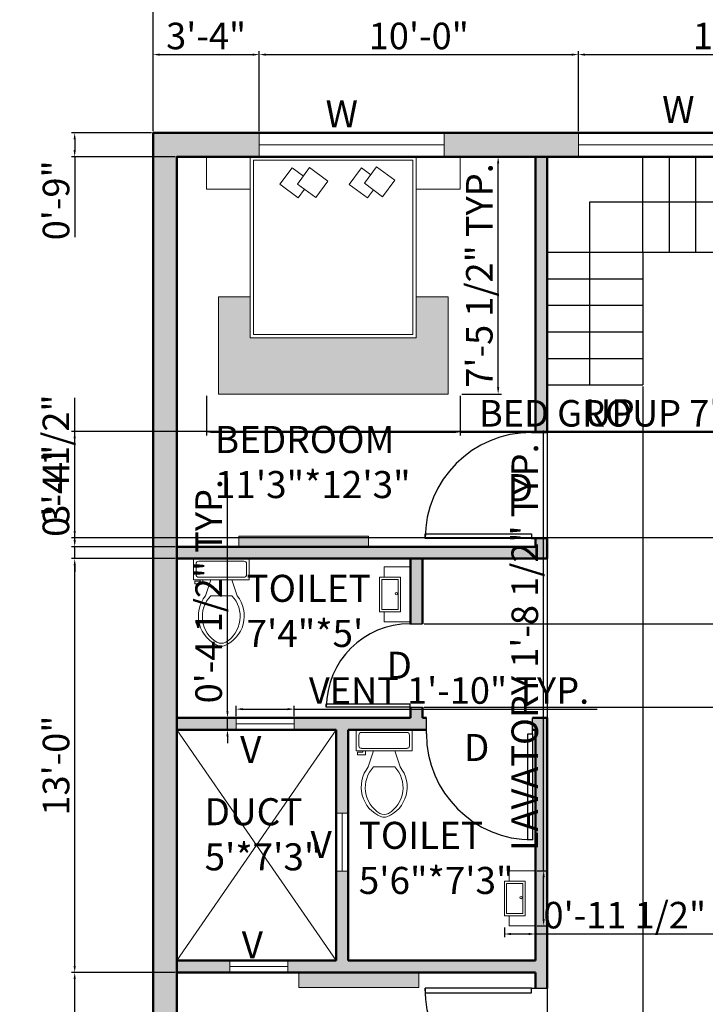
# Model space of a CAD drawing. Units: inches. Extents: x 1822 to 2392, y 2066 to 2908.
# Tile 2 of 4: x 1822 to 2080, y 2256 to 2627. Entities that reach past the tile are written whole.
import ezdxf

# ---------------------------------------------------------------- set-up
doc = ezdxf.new("R2010")
doc.units = ezdxf.units.IN
for name, color, linetype, lineweight in [('A-ANNO-DIMS', 2, 'Continuous', 18), ('A-AREA-IDEN', 83, 'Continuous', 25), ('A-EQPM-PATT', 89, 'Continuous', 13), ('A-FLOR-OPEN', 8, 'Continuous', 18), ('A-FLOR-PATT', 9, 'Continuous', 13), ('A-WALL-PATT', 252, 'Continuous', 13), ('BEDS', 40, 'Continuous', 18), ('DOOR', 50, 'Continuous', 25), ('STAIR', 32, 'Continuous', 25), ('TEXT', 83, 'Continuous', 25), ('TOILET', 220, 'Continuous', 18), ('TV', 89, 'Continuous', 18), ('wall', 7, 'Continuous', 50), ('WINDOW', 80, 'Continuous', 20)]:
    doc.layers.add(name, color=color, linetype=linetype, lineweight=lineweight)
doc.styles.get("Standard").update_dxf_attribs({"font": 'arial.ttf'})
doc.dimstyles.new('ISO-25', dxfattribs={"dimtxt": 10, "dimasz": 2.5, "dimexe": 1.25, "dimexo": 0.625, "dimtad": 1, "dimdec": 0, "dimlunit": 4, "dimtxsty": 'Standard', "dimcen": 2.5, "dimadec": 0, "dimazin": 0, "dimtfac": 1, "dimtdec": 0, "dimtmove": 0, "dimatfit": 3, "dimfxl": 1, "dimarcsym": 0})

# ---------------------------------------------------------------- blocks, each defined once
blk = doc.blocks.new('*U2')
for p, q in [((0, 0), (0, -6)), ((40, 0), (40, -6))]:
    blk.add_line(p, q)
blk.add_lwpolyline([(0, 0), (0, 40), (1.75, 40), (1.75, 0)], close=True)
blk.add_arc((0, 0), 40, 0, 90)
blk = doc.blocks.new('*U4')
for p, q in [((9.5, -6), (9.5, -2)), ((-10, -8.5), (-8, -8.5)), ((-10, -9.5), (-10, -8.5)), ((-7, -9.5), (-10, -9.5)), ((-8, -8.5), (-8, -8)), ((-7, -8), (-7, -9.5)), ((-4, -8), (-6, -14)), ((4, -8), (6, -14)), ((4, -14), (-4, -14))]:
    blk.add_line(p, q)
blk.add_lwpolyline([(10.5, -8), (10.5, 0), (-10.5, 0), (-10.5, -8)], close=True)
for points in [[(-9.5, -2), (-9.5, -6)], [(8.5, -1), (-8.5, -1)], [(-8.5, -7), (8.5, -7)]]:
    blk.add_lwpolyline(points)
for centre, radius, start, end in [((-8.62, -1.88), 0.884, 81.8699, 188.1301), ((8.62, -1.88), 0.884, 351.8699, 98.1301), ((-8.62, -6.12), 0.884, 171.8699, 278.1301), ((8.62, -6.12), 0.884, 261.8699, 8.1301), ((3.52, -21.58), 12.17, 141.4691, 247.9714), ((4.2, -21.82), 11.33, 136.3677, 238.9468), ((-3.52, -21.58), 12.17, 292.0284, 38.5307), ((-4.2, -21.82), 11.33, 301.053, 43.6321), ((0, -27.88), 4, 245.7318, 294.2682), ((0, -29), 4, 254.8605, 285.1395)]:
    blk.add_arc(centre, radius, start, end)
blk = doc.blocks.new('*D5')
at = {"layer": 'A-ANNO-DIMS', "color": 0, "lineweight": -2, "transparency": 16777216}
for p, q in [((1872.41, 2584.74), (1872.41, 2632.85)), ((1874.91, 2631.6), (2265.91, 2631.6)), ((2268.41, 2584.74), (2268.41, 2632.85))]:
    blk.add_line(p, q, dxfattribs=at)
at = {"layer": 'A-ANNO-DIMS', "color": 0, "transparency": 16777216}
for points in [[(1874.91, 2632.01), (1874.91, 2631.18), (1872.41, 2631.6)], [(2265.91, 2632.01), (2265.91, 2631.18), (2268.41, 2631.6)]]:
    blk.add_solid(points, dxfattribs=at)
at = {"layer": 'Defpoints', "color": 0, "transparency": 16777216}
for p in [(2268.41, 2631.6), (1872.41, 2584.12), (2268.41, 2584.12)]:
    blk.add_point(p, dxfattribs=at)
at = {"layer": 'A-ANNO-DIMS', "color": 0, "transparency": 16777216, "insert": (2070.41, 2637.33), "char_height": 10, "attachment_point": 5}
blk.add_mtext("33'", dxfattribs=at)
blk = doc.blocks.new('BED-DOUBLE-WITH-NIGHTSTANDS')
for p, q in [((0, -52.84), (-12, -52.84)), ((-12, -52.84), (-12, -89.47)), ((62.55, -52.84), (74.55, -52.84)), ((74.55, -52.84), (74.55, -89.47)), ((-12, -89.47), (74.55, -89.47))]:
    blk.add_line(p, q)
for points in [[(0, 0), (-16.5, 0), (-16.5, -12.19), (0, -12.19)], [(0, 0), (62.55, 0), (62.55, -68.27), (0, -68.27)], [(79.04, 0), (62.55, 0), (62.55, -12.19), (79.04, -12.19)], [(1.28, -1.28), (61.27, -1.28), (61.27, -67), (1.28, -67)], [(22.38, -4.1), (29.25, -9.19), (24.65, -15.4), (17.78, -10.31)], [(47.61, -3.78), (54.48, -8.87), (49.87, -15.08), (43, -9.99)]]:
    blk.add_lwpolyline(points, close=True)
for points in [[(20.42, -12.27), (18.06, -15.45), (11.2, -10.36), (15.8, -4.15), (20.02, -7.28)], [(46.41, -12.52), (44.19, -15.51), (37.32, -10.42), (41.93, -4.21), (45.39, -6.77)]]:
    blk.add_lwpolyline(points)
blk = doc.blocks.new('LAVATORY-WALL-MOUNT')
for p, q in [((1.78, 16.83), (1.78, 20.72)), ((1.78, 20.72), (11.67, 20.72)), ((1.78, 3.73), (1.78, 0)), ((1.78, 0), (11.67, 0))]:
    blk.add_line(p, q)
for points in [[(7.82, 16.83), (0, 16.83), (0, 3.73), (7.82, 3.73)], [(6.96, 15.97), (0.86, 15.97), (0.86, 4.59), (6.96, 4.59)]]:
    blk.add_lwpolyline(points, close=True)
blk.add_circle((6.29, 10.59), 0.446)
blk = doc.blocks.new('WINDOW-EXT-TYPE-A')
blk.add_line((0, 4.5), (69.61, 4.5))
blk.add_lwpolyline([(0, 9), (69.61, 9), (69.61, 0), (0, 0)], close=True)
blk = doc.blocks.new('VENT-INT-TYPE-A')
blk.add_line((0, 2.25), (21.86, 2.25))
blk.add_lwpolyline([(0, 4.5), (21.86, 4.5), (21.86, 0), (0, 0)], close=True)
blk = doc.blocks.new('TV-BEDROOM-TYPE-A')
blk.add_lwpolyline([(0, 0), (48.81, 0), (48.81, 3.94), (0, 3.94)], close=True)
blk = doc.blocks.new('*D16')
at = {"layer": 'A-ANNO-DIMS', "color": 0, "lineweight": -2, "transparency": 16777216}
for p, q in [((1892.52, 2485.02), (1892.52, 2470.06)), ((1988.06, 2485.02), (1988.06, 2470.06)), ((1895.02, 2471.31), (1985.56, 2471.31)), ((1988.06, 2471.31), (2171.11, 2471.31))]:
    blk.add_line(p, q, dxfattribs=at)
at = {"layer": 'A-ANNO-DIMS', "color": 0, "transparency": 16777216}
for points in [[(1895.02, 2471.73), (1895.02, 2470.9), (1892.52, 2471.31)], [(1985.56, 2471.73), (1985.56, 2470.9), (1988.06, 2471.31)]]:
    blk.add_solid(points, dxfattribs=at)
at = {"layer": 'Defpoints', "color": 0, "transparency": 16777216}
for p in [(1892.52, 2485.65), (1988.06, 2485.65), (1988.06, 2471.31)]:
    blk.add_point(p, dxfattribs=at)
at = {"layer": 'A-ANNO-DIMS', "color": 0, "transparency": 16777216, "insert": (2080.84, 2477.11), "char_height": 10, "attachment_point": 5}
blk.add_mtext('BED GROUP 7\'-11 1/2" TYP.', dxfattribs=at)
blk = doc.blocks.new('*D17')
at = {"layer": 'A-ANNO-DIMS', "color": 0, "lineweight": -2, "transparency": 16777216}
for p, q in [((1988.69, 2575.12), (2003.64, 2575.12)), ((2002.39, 2488.15), (2002.39, 2572.62)), ((1988.69, 2485.65), (2003.64, 2485.65))]:
    blk.add_line(p, q, dxfattribs=at)
at = {"layer": 'A-ANNO-DIMS', "color": 0, "transparency": 16777216}
for points in [[(2001.98, 2572.62), (2002.81, 2572.62), (2002.39, 2575.12)], [(2001.98, 2488.15), (2002.81, 2488.15), (2002.39, 2485.65)]]:
    blk.add_solid(points, dxfattribs=at)
at = {"layer": 'Defpoints', "color": 0, "transparency": 16777216}
for p in [(1988.06, 2575.12), (2002.39, 2575.12), (1988.06, 2485.65)]:
    blk.add_point(p, dxfattribs=at)
at = {"layer": 'A-ANNO-DIMS', "color": 0, "transparency": 16777216, "insert": (1996.6, 2530.38), "char_height": 10, "attachment_point": 5, "rotation": 90}
blk.add_mtext('7\'-5 1/2" TYP.', dxfattribs=at)
blk = doc.blocks.new('*D20')
at = {"layer": 'A-ANNO-DIMS', "color": 0, "lineweight": -2, "transparency": 16777216}
for p, q in [((1903.72, 2364.24), (1903.72, 2368.15)), ((1925.58, 2364.24), (1925.58, 2368.15)), ((1906.22, 2366.9), (1923.08, 2366.9)), ((1925.58, 2366.9), (2039.72, 2366.9))]:
    blk.add_line(p, q, dxfattribs=at)
at = {"layer": 'A-ANNO-DIMS', "color": 0, "transparency": 16777216}
for points in [[(1906.22, 2367.31), (1906.22, 2366.48), (1903.72, 2366.9)], [(1923.08, 2367.31), (1923.08, 2366.48), (1925.58, 2366.9)]]:
    blk.add_solid(points, dxfattribs=at)
at = {"layer": 'Defpoints', "color": 0, "transparency": 16777216}
for p in [(1925.58, 2366.9), (1903.72, 2363.62), (1925.58, 2363.62)]:
    blk.add_point(p, dxfattribs=at)
at = {"layer": 'A-ANNO-DIMS', "color": 0, "transparency": 16777216, "insert": (1983.9, 2372.63), "char_height": 10, "attachment_point": 5}
blk.add_mtext('VENT 1\'-10" TYP.', dxfattribs=at)
blk = doc.blocks.new('*D21')
at = {"layer": 'A-ANNO-DIMS', "color": 0, "lineweight": -2, "transparency": 16777216}
for p, q in [((1900.45, 2366.12), (1900.45, 2454.12)), ((1903.1, 2363.62), (1899.2, 2363.62)), ((1900.45, 2359.12), (1900.45, 2363.62)), ((1903.1, 2359.12), (1899.2, 2359.12)), ((1900.45, 2356.62), (1900.45, 2354.12))]:
    blk.add_line(p, q, dxfattribs=at)
at = {"layer": 'A-ANNO-DIMS', "color": 0, "transparency": 16777216}
for points in [[(1900.03, 2366.12), (1900.86, 2366.12), (1900.45, 2363.62)], [(1900.03, 2356.62), (1900.86, 2356.62), (1900.45, 2359.12)]]:
    blk.add_solid(points, dxfattribs=at)
at = {"layer": 'Defpoints', "color": 0, "transparency": 16777216}
for p in [(1900.45, 2363.62), (1903.72, 2363.62), (1903.72, 2359.12)]:
    blk.add_point(p, dxfattribs=at)
at = {"layer": 'A-ANNO-DIMS', "color": 0, "transparency": 16777216, "insert": (1894.65, 2411.37), "char_height": 10, "attachment_point": 5, "rotation": 90}
blk.add_mtext('0\'-4 1/2" TYP.', dxfattribs=at)
blk = doc.blocks.new('*D22')
at = {"layer": 'A-ANNO-DIMS', "color": 0, "lineweight": -2, "transparency": 16777216}
for p, q in [((2019.52, 2305.97), (2019.52, 2471.95)), ((2017.04, 2305.97), (2020.77, 2305.97)), ((2019.52, 2287.75), (2019.52, 2303.47)), ((2017.04, 2285.25), (2020.77, 2285.25))]:
    blk.add_line(p, q, dxfattribs=at)
at = {"layer": 'A-ANNO-DIMS', "color": 0, "transparency": 16777216}
for points in [[(2019.1, 2303.47), (2019.94, 2303.47), (2019.52, 2305.97)], [(2019.1, 2287.75), (2019.94, 2287.75), (2019.52, 2285.25)]]:
    blk.add_solid(points, dxfattribs=at)
at = {"layer": 'Defpoints', "color": 0, "transparency": 16777216}
for p in [(2016.41, 2305.97), (2019.52, 2305.97), (2016.41, 2285.25)]:
    blk.add_point(p, dxfattribs=at)
at = {"layer": 'A-ANNO-DIMS', "color": 0, "transparency": 16777216, "insert": (2013.72, 2390.21), "char_height": 10, "attachment_point": 5, "rotation": 90}
blk.add_mtext('LAVATORY 1\'-8 1/2" TYP.', dxfattribs=at)
blk = doc.blocks.new('*D23')
at = {"layer": 'A-ANNO-DIMS', "color": 0, "lineweight": -2, "transparency": 16777216}
for p, q in [((2004.74, 2284.62), (2004.74, 2280.89)), ((2016.41, 2284.62), (2016.41, 2280.89)), ((2007.24, 2282.14), (2013.91, 2282.14)), ((2016.41, 2282.14), (2112.19, 2282.14))]:
    blk.add_line(p, q, dxfattribs=at)
at = {"layer": 'A-ANNO-DIMS', "color": 0, "transparency": 16777216}
for points in [[(2007.24, 2282.56), (2007.24, 2281.73), (2004.74, 2282.14)], [(2013.91, 2282.56), (2013.91, 2281.73), (2016.41, 2282.14)]]:
    blk.add_solid(points, dxfattribs=at)
at = {"layer": 'Defpoints', "color": 0, "transparency": 16777216}
for p in [(2004.74, 2285.25), (2016.41, 2285.25), (2016.41, 2282.14)]:
    blk.add_point(p, dxfattribs=at)
at = {"layer": 'A-ANNO-DIMS', "color": 0, "transparency": 16777216, "insert": (2065.55, 2287.94), "char_height": 10, "attachment_point": 5}
blk.add_mtext('0\'-11 1/2" TYP.', dxfattribs=at)
blk = doc.blocks.new('*D28')
at = {"layer": 'A-ANNO-DIMS', "color": 0, "lineweight": -2, "transparency": 16777216}
for p, q in [((1872.41, 2584.74), (1872.41, 2614.87)), ((1874.91, 2613.62), (1909.9, 2613.62)), ((1912.4, 2584.74), (1912.4, 2614.87))]:
    blk.add_line(p, q, dxfattribs=at)
at = {"layer": 'A-ANNO-DIMS', "color": 0, "transparency": 16777216}
for points in [[(1874.91, 2614.03), (1874.91, 2613.2), (1872.41, 2613.62)], [(1909.9, 2614.03), (1909.9, 2613.2), (1912.4, 2613.62)]]:
    blk.add_solid(points, dxfattribs=at)
at = {"layer": 'Defpoints', "color": 0, "transparency": 16777216}
for p in [(1912.4, 2613.62), (1872.41, 2584.12), (1912.4, 2584.12)]:
    blk.add_point(p, dxfattribs=at)
at = {"layer": 'A-ANNO-DIMS', "color": 0, "transparency": 16777216, "insert": (1892.41, 2619.35), "char_height": 10, "attachment_point": 5}
blk.add_mtext('3\'-4"', dxfattribs=at)
blk = doc.blocks.new('*D29')
at = {"layer": 'A-ANNO-DIMS', "color": 0, "lineweight": -2, "transparency": 16777216}
for p, q in [((1912.4, 2584.74), (1912.4, 2614.87)), ((1914.9, 2613.62), (2030.12, 2613.62)), ((2032.62, 2584.74), (2032.62, 2614.87))]:
    blk.add_line(p, q, dxfattribs=at)
at = {"layer": 'A-ANNO-DIMS', "color": 0, "transparency": 16777216}
for points in [[(1914.9, 2614.03), (1914.9, 2613.2), (1912.4, 2613.62)], [(2030.12, 2614.03), (2030.12, 2613.2), (2032.62, 2613.62)]]:
    blk.add_solid(points, dxfattribs=at)
at = {"layer": 'Defpoints', "color": 0, "transparency": 16777216}
for p in [(2032.62, 2613.62), (1912.4, 2584.12), (2032.62, 2584.12)]:
    blk.add_point(p, dxfattribs=at)
at = {"layer": 'A-ANNO-DIMS', "color": 0, "transparency": 16777216, "insert": (1972.51, 2619.35), "char_height": 10, "attachment_point": 5}
blk.add_mtext('10\'-0"', dxfattribs=at)
blk = doc.blocks.new('*D30')
at = {"layer": 'A-ANNO-DIMS', "color": 0, "lineweight": -2, "transparency": 16777216}
for p, q in [((2032.62, 2584.74), (2032.62, 2614.87)), ((2035.12, 2613.62), (2154.11, 2613.62)), ((2156.61, 2584.74), (2156.61, 2614.87))]:
    blk.add_line(p, q, dxfattribs=at)
at = {"layer": 'A-ANNO-DIMS', "color": 0, "transparency": 16777216}
for points in [[(2035.12, 2614.03), (2035.12, 2613.2), (2032.62, 2613.62)], [(2154.11, 2614.03), (2154.11, 2613.2), (2156.61, 2613.62)]]:
    blk.add_solid(points, dxfattribs=at)
at = {"layer": 'Defpoints', "color": 0, "transparency": 16777216}
for p in [(2156.61, 2613.62), (2032.62, 2584.12), (2156.61, 2584.12)]:
    blk.add_point(p, dxfattribs=at)
at = {"layer": 'A-ANNO-DIMS', "color": 0, "transparency": 16777216, "insert": (2094.62, 2619.35), "char_height": 10, "attachment_point": 5}
blk.add_mtext('10\'-4"', dxfattribs=at)
blk = doc.blocks.new('*D39')
at = {"layer": 'A-ANNO-DIMS', "color": 0, "lineweight": -2, "transparency": 16777216}
for p, q in [((1871.79, 2584.12), (1841.66, 2584.12)), ((1842.91, 2581.62), (1842.91, 2577.62)), ((1880.79, 2575.12), (1841.66, 2575.12)), ((1842.91, 2575.12), (1842.91, 2544.78))]:
    blk.add_line(p, q, dxfattribs=at)
at = {"layer": 'A-ANNO-DIMS', "color": 0, "transparency": 16777216}
for points in [[(1842.5, 2581.62), (1843.33, 2581.62), (1842.91, 2584.12)], [(1842.5, 2577.62), (1843.33, 2577.62), (1842.91, 2575.12)]]:
    blk.add_solid(points, dxfattribs=at)
at = {"layer": 'Defpoints', "color": 0, "transparency": 16777216}
for p in [(1872.41, 2584.12), (1842.91, 2575.12), (1881.41, 2575.12)]:
    blk.add_point(p, dxfattribs=at)
at = {"layer": 'A-ANNO-DIMS', "color": 0, "transparency": 16777216, "insert": (1837.18, 2558.7), "char_height": 10, "attachment_point": 5, "rotation": 90}
blk.add_mtext('0\'-9"', dxfattribs=at)
blk = doc.blocks.new('*D40')
at = {"layer": 'A-ANNO-DIMS', "color": 0, "lineweight": -2, "transparency": 16777216}
for p, q in [((1842.91, 2430.62), (1842.91, 2484.25)), ((1880.79, 2428.12), (1841.66, 2428.12)), ((1842.91, 2423.62), (1842.91, 2428.12)), ((1880.79, 2423.62), (1841.66, 2423.62)), ((1842.91, 2421.12), (1842.91, 2418.62))]:
    blk.add_line(p, q, dxfattribs=at)
at = {"layer": 'A-ANNO-DIMS', "color": 0, "transparency": 16777216}
for points in [[(1842.5, 2430.62), (1843.33, 2430.62), (1842.91, 2428.12)], [(1842.5, 2421.12), (1843.33, 2421.12), (1842.91, 2423.62)]]:
    blk.add_solid(points, dxfattribs=at)
at = {"layer": 'Defpoints', "color": 0, "transparency": 16777216}
for p in [(1842.91, 2428.12), (1881.41, 2428.12), (1881.41, 2423.62)]:
    blk.add_point(p, dxfattribs=at)
at = {"layer": 'A-ANNO-DIMS', "color": 0, "transparency": 16777216, "insert": (1837.12, 2458.68), "char_height": 10, "attachment_point": 5, "rotation": 90}
blk.add_mtext('0\'-4 1/2"', dxfattribs=at)
blk = doc.blocks.new('*D41')
at = {"layer": 'A-ANNO-DIMS', "color": 0, "lineweight": -2, "transparency": 16777216}
for p, q in [((2020.91, 2488.49), (2020.91, 2073.37)), ((2056.91, 2488.49), (2056.91, 2073.37)), ((2023.41, 2074.62), (2054.41, 2074.62))]:
    blk.add_line(p, q, dxfattribs=at)
at = {"layer": 'A-ANNO-DIMS', "color": 0, "transparency": 16777216}
for points in [[(2023.41, 2075.03), (2023.41, 2074.2), (2020.91, 2074.62)], [(2054.41, 2075.03), (2054.41, 2074.2), (2056.91, 2074.62)]]:
    blk.add_solid(points, dxfattribs=at)
at = {"layer": 'Defpoints', "color": 0, "transparency": 16777216}
for p in [(2020.91, 2489.12), (2056.91, 2489.12), (2056.91, 2074.62)]:
    blk.add_point(p, dxfattribs=at)
at = {"layer": 'A-ANNO-DIMS', "color": 0, "transparency": 16777216, "insert": (2038.91, 2080.35), "char_height": 10, "attachment_point": 5}
blk.add_mtext('3\'-0"', dxfattribs=at)
blk = doc.blocks.new('*D43')
at = {"layer": 'A-ANNO-DIMS', "color": 0, "lineweight": -2, "transparency": 16777216}
for p, q in [((2119.29, 2471.52), (1841.66, 2471.52)), ((1842.91, 2434.02), (1842.91, 2469.02)), ((2119.29, 2431.52), (1841.66, 2431.52))]:
    blk.add_line(p, q, dxfattribs=at)
at = {"layer": 'A-ANNO-DIMS', "color": 0, "transparency": 16777216}
for points in [[(1842.5, 2469.02), (1843.33, 2469.02), (1842.91, 2471.52)], [(1842.5, 2434.02), (1843.33, 2434.02), (1842.91, 2431.52)]]:
    blk.add_solid(points, dxfattribs=at)
at = {"layer": 'Defpoints', "color": 0, "transparency": 16777216}
for p in [(1842.91, 2471.52), (2119.91, 2471.52), (2119.91, 2431.52)]:
    blk.add_point(p, dxfattribs=at)
at = {"layer": 'A-ANNO-DIMS', "color": 0, "transparency": 16777216, "insert": (1837.18, 2451.52), "char_height": 10, "attachment_point": 5, "rotation": 90}
blk.add_mtext('3\'-4"', dxfattribs=at)
blk = doc.blocks.new('*D44')
at = {"layer": 'A-ANNO-DIMS', "color": 0, "lineweight": -2, "transparency": 16777216}
for p, q in [((2297.91, 2399.09), (2297.91, 2452.89)), ((1974.54, 2399.09), (2299.16, 2399.09)), ((2297.91, 2370.08), (2297.91, 2396.59)), ((1974.54, 2367.58), (2299.16, 2367.58))]:
    blk.add_line(p, q, dxfattribs=at)
at = {"layer": 'A-ANNO-DIMS', "color": 0, "transparency": 16777216}
for points in [[(2297.5, 2396.59), (2298.33, 2396.59), (2297.91, 2399.09)], [(2297.5, 2370.08), (2298.33, 2370.08), (2297.91, 2367.58)]]:
    blk.add_solid(points, dxfattribs=at)
at = {"layer": 'Defpoints', "color": 0, "transparency": 16777216}
for p in [(1973.91, 2399.09), (2297.91, 2399.09), (1973.91, 2367.58)]:
    blk.add_point(p, dxfattribs=at)
at = {"layer": 'A-ANNO-DIMS', "color": 0, "transparency": 16777216, "insert": (2292.12, 2427.24), "char_height": 10, "attachment_point": 5, "rotation": 90}
blk.add_mtext('2\'-7 1/2"', dxfattribs=at)
blk = doc.blocks.new('*D46')
at = {"layer": 'A-ANNO-DIMS', "color": 0, "lineweight": -2, "transparency": 16777216}
for p, q in [((1880.79, 2267.62), (1841.66, 2267.62)), ((1842.91, 2106.62), (1842.91, 2265.12)), ((1871.79, 2104.12), (1841.66, 2104.12))]:
    blk.add_line(p, q, dxfattribs=at)
at = {"layer": 'A-ANNO-DIMS', "color": 0, "transparency": 16777216}
for points in [[(1842.5, 2265.12), (1843.33, 2265.12), (1842.91, 2267.62)], [(1842.5, 2106.62), (1843.33, 2106.62), (1842.91, 2104.12)]]:
    blk.add_solid(points, dxfattribs=at)
at = {"layer": 'Defpoints', "color": 0, "transparency": 16777216}
for p in [(1842.91, 2267.62), (1881.41, 2267.62), (1872.41, 2104.12)]:
    blk.add_point(p, dxfattribs=at)
at = {"layer": 'A-ANNO-DIMS', "color": 0, "transparency": 16777216, "insert": (1837.11, 2185.87), "char_height": 10, "attachment_point": 5, "rotation": 90}
blk.add_mtext('13\'-7 1/2"', dxfattribs=at)
blk = doc.blocks.new('*D47')
at = {"layer": 'A-ANNO-DIMS', "color": 0, "lineweight": -2, "transparency": 16777216}
for p, q in [((1880.79, 2423.62), (1841.66, 2423.62)), ((1842.91, 2270.12), (1842.91, 2421.12)), ((1880.79, 2267.62), (1841.66, 2267.62))]:
    blk.add_line(p, q, dxfattribs=at)
at = {"layer": 'A-ANNO-DIMS', "color": 0, "transparency": 16777216}
for points in [[(1842.5, 2421.12), (1843.33, 2421.12), (1842.91, 2423.62)], [(1842.5, 2270.12), (1843.33, 2270.12), (1842.91, 2267.62)]]:
    blk.add_solid(points, dxfattribs=at)
at = {"layer": 'Defpoints', "color": 0, "transparency": 16777216}
for p in [(1842.91, 2423.62), (1881.41, 2423.62), (1881.41, 2267.62)]:
    blk.add_point(p, dxfattribs=at)
at = {"layer": 'A-ANNO-DIMS', "color": 0, "transparency": 16777216, "insert": (1837.18, 2345.62), "char_height": 10, "attachment_point": 5, "rotation": 90}
blk.add_mtext('13\'-0"', dxfattribs=at)

msp = doc.modelspace()

# ---------------------------------------------------------------- hatches: boundary and pattern name
at = {"layer": 'A-EQPM-PATT'}
h = msp.add_hatch(color=256, dxfattribs=at)
h.dxf.hatch_style = 1
h.paths.add_polyline_path([(2259.41, 2352.89), (2253.4, 2352.89), (2253.4, 2300.49), (2259.41, 2300.49)])
h.paths.add_polyline_path([(1972.53, 2267.62), (1927.37, 2267.62), (1927.37, 2261.95), (1972.53, 2261.95)])
h.paths.add_polyline_path([(1953.54, 2432.06), (1904.73, 2432.06), (1904.73, 2428.12), (1953.54, 2428.12)])
at = {"layer": 'A-FLOR-PATT'}
h = msp.add_hatch(dxfattribs=at)
h.set_pattern_fill('ANSI36', color=256)
h.paths.add_polyline_path([(1983.57, 2522.27), (1971.57, 2522.27), (1971.57, 2506.84), (1909.02, 2506.84), (1909.02, 2522.27), (1897.02, 2522.27), (1897.02, 2485.65), (1983.57, 2485.65)])
h.paths.add_polyline_path([(1988.24, 2202.59), (1901.7, 2202.59), (1901.7, 2165.96), (1913.7, 2165.96), (1913.7, 2181.39), (1976.24, 2181.39), (1976.24, 2165.96), (1988.24, 2165.96)])
h.paths.add_polyline_path([(2250.08, 2522.27), (2238.08, 2522.27), (2238.08, 2506.84), (2175.53, 2506.84), (2175.53, 2522.27), (2163.53, 2522.27), (2163.53, 2485.65), (2250.08, 2485.65)])
at = {"layer": 'A-WALL-PATT'}
h = msp.add_hatch(color=256, dxfattribs=at)
h.dxf.hatch_style = 1
h.paths.add_polyline_path([(2032.62, 2584.12), (1982.01, 2584.12), (1982.01, 2575.12), (1988.06, 2575.12), (2016.41, 2575.12), (2032.62, 2575.12)], flags=17)
h.paths.add_polyline_path([(2156.61, 2584.12), (2102.23, 2584.12), (2102.23, 2575.12), (2119.91, 2575.12), (2156.61, 2575.12)], flags=17)
h.paths.add_polyline_path([(1914.42, 2104.12), (1914.42, 2113.12), (1881.41, 2113.12), (1881.41, 2575.12), (1912.4, 2575.12), (1912.4, 2584.12), (1872.41, 2584.12), (1872.41, 2104.12)])
h.paths.add_polyline_path([(2268.41, 2129.27), (2259.41, 2129.27), (2259.41, 2113.12), (2224.8, 2113.12), (2224.8, 2104.12), (2268.41, 2104.12)])
h.paths.add_polyline_path([(2268.41, 2236.1), (2259.41, 2236.1), (2259.41, 2198.88), (2268.41, 2198.88)])
h.paths.add_polyline_path([(2268.41, 2358.32), (2259.41, 2358.32), (2259.41, 2292.4), (2268.41, 2292.4)])
h.paths.add_polyline_path([(2259.41, 2554.73), (2268.41, 2554.73), (2268.41, 2584.12), (2226.22, 2584.12), (2226.22, 2575.12), (2259.41, 2575.12)])
h.paths.add_polyline_path([(2268.41, 2485.12), (2259.41, 2485.12), (2259.41, 2408.76), (2268.41, 2408.76)])
h.paths.add_polyline_path([(2020.91, 2104.12), (2020.91, 2113.12), (1984.03, 2113.12), (1984.03, 2104.12)])
h.paths.add_polyline_path([(2119.91, 2113.12), (2119.91, 2104.12), (2155.19, 2104.12), (2155.19, 2113.12)])
h = msp.add_hatch(color=256, dxfattribs=at)
h.dxf.hatch_style = 1
h.paths.add_polyline_path([(2124.41, 2575.12), (2119.91, 2575.12), (2119.91, 2471.52), (2124.41, 2471.52)])
h.paths.add_polyline_path([(2020.91, 2575.12), (2016.41, 2575.12), (2016.41, 2471.18), (2020.91, 2471.18)])
h.paths.add_polyline_path([(2259.41, 2428.12), (2124.41, 2428.12), (2124.41, 2431.52), (2119.91, 2431.52), (2119.91, 2423.62), (2259.41, 2423.62)])
h.paths.add_polyline_path([(2020.91, 2363.62), (2016.41, 2363.62), (2015.38, 2363.62), (2015.38, 2359.12), (2016.41, 2359.12), (2016.41, 2272.12), (1945.91, 2272.12), (1945.91, 2305.88), (1941.41, 2305.88), (1941.41, 2272.12), (1923.14, 2272.12), (1923.14, 2267.62), (2016.41, 2267.62), (2016.41, 2261.67), (2020.91, 2261.67), (2020.91, 2267.62)])
h.paths.add_polyline_path([(2259.41, 2213.62), (2168.4, 2213.62), (2168.4, 2209.12), (2259.41, 2209.12)])
h.paths.add_polyline_path([(2124.41, 2209.12), (2128.4, 2209.12), (2128.4, 2213.62), (2119.91, 2213.62), (2119.91, 2113.12), (2124.41, 2113.12), (2124.41, 2137.12)])
h.paths.add_polyline_path([(2020.91, 2221.67), (2016.41, 2221.67), (2016.41, 2113.12), (2020.91, 2113.12), (2020.91, 2137.12)])
h.paths.add_polyline_path([(2034.48, 2141.62), (2020.91, 2141.62), (2020.91, 2137.12), (2034.48, 2137.12)])
h.paths.add_polyline_path([(2119.91, 2141.62), (2102.28, 2141.62), (2102.28, 2137.12), (2119.91, 2137.12)])
h.paths.add_polyline_path([(1973.91, 2423.62), (1969.41, 2423.62), (1969.41, 2399.09), (1973.91, 2399.09)])
h = msp.add_hatch(color=256, dxfattribs=at)
h.dxf.hatch_style = 1
h.paths.add_polyline_path([(2020.91, 2431.18), (2016.41, 2431.18), (2016.41, 2428.12), (1881.41, 2428.12), (1881.41, 2423.62), (2020.91, 2423.62)])
h.paths.add_polyline_path([(1975.38, 2363.62), (1973.91, 2363.62), (1973.91, 2367.58), (1969.41, 2367.58), (1969.41, 2363.62), (1925.58, 2363.62), (1925.58, 2359.12), (1941.41, 2359.12), (1941.41, 2327.74), (1945.91, 2327.74), (1945.91, 2359.12), (1975.38, 2359.12)])
h.paths.add_polyline_path([(1903.72, 2363.62), (1881.41, 2363.62), (1881.41, 2359.12), (1903.72, 2359.12)])
h.paths.add_polyline_path([(1901.28, 2272.12), (1881.41, 2272.12), (1881.41, 2267.62), (1901.28, 2267.62)])

# ---------------------------------------------------------------- linework, layer by layer
at = {"layer": 'A-FLOR-OPEN'}
for p, q in [((1881.41, 2272.12), (1941.41, 2359.12)), ((1881.41, 2359.12), (1941.41, 2272.12))]:
    msp.add_line(p, q, dxfattribs=at)
at = {"layer": 'STAIR'}
for p, q in [((2020.91, 2575.12), (2020.91, 2539.12)), ((2020.91, 2575.12), (2056.91, 2575.12)), ((2056.91, 2539.12), (2056.91, 2575.12)), ((2066.91, 2539.12), (2066.91, 2575.12)), ((2076.91, 2539.12), (2076.91, 2575.12)), ((2036.89, 2489.12), (2036.89, 2558.17)), ((2036.89, 2558.17), (2104.24, 2558.17)), ((2020.91, 2539.12), (2056.91, 2539.12)), ((2056.91, 2539.12), (2056.91, 2489.12)), ((2056.91, 2539.12), (2083.91, 2539.12)), ((2020.91, 2529.12), (2056.91, 2529.12)), ((2020.91, 2519.12), (2056.91, 2519.12)), ((2020.91, 2509.12), (2056.91, 2509.12)), ((2020.91, 2499.12), (2056.91, 2499.12)), ((2020.91, 2489.12), (2056.91, 2489.12))]:
    msp.add_line(p, q, dxfattribs=at)
at = {"layer": 'TV'}
msp.add_lwpolyline([(1927.37, 2267.62), (1972.53, 2267.62), (1972.53, 2261.95), (1927.37, 2261.95)], close=True, dxfattribs=at)
at = {"layer": 'wall'}
for p, q in [((1881.41, 2575.12), (2016.41, 2575.12)), ((2016.41, 2575.12), (2016.41, 2471.18)), ((2020.91, 2575.12), (2020.91, 2471.18)), ((2016.41, 2431.18), (2016.41, 2428.12)), ((2020.91, 2431.18), (2020.91, 2423.62)), ((2016.41, 2428.12), (1881.41, 2428.12)), ((2020.91, 2423.62), (1881.41, 2423.62)), ((1881.41, 2423.62), (1881.41, 2363.62)), ((1969.41, 2399.09), (1969.41, 2423.62)), ((1973.91, 2399.09), (1973.91, 2423.62)), ((1969.41, 2363.62), (1969.41, 2367.58)), ((1973.91, 2363.62), (1973.91, 2367.58)), ((1881.41, 2363.62), (1969.41, 2363.62)), ((1945.91, 2363.62), (1969.41, 2363.62)), ((1973.91, 2363.62), (1975.38, 2363.62)), ((2015.38, 2363.62), (2016.41, 2363.62)), ((2016.41, 2363.62), (2020.91, 2363.62)), ((2020.91, 2363.62), (2020.91, 2267.62)), ((1881.41, 2359.12), (1941.41, 2359.12)), ((1881.41, 2359.12), (1941.41, 2359.12)), ((1941.41, 2359.12), (1941.41, 2272.12)), ((1945.91, 2359.12), (1945.91, 2272.12)), ((1945.91, 2359.12), (1975.38, 2359.12)), ((1945.91, 2359.12), (1973.91, 2359.12)), ((2015.38, 2359.12), (2016.41, 2359.12)), ((2016.41, 2359.12), (2016.41, 2272.12)), ((1941.41, 2272.12), (1881.41, 2272.12)), ((2016.41, 2272.12), (1945.91, 2272.12)), ((1945.91, 2267.62), (1881.41, 2267.62)), ((1881.41, 2267.62), (1881.41, 2126.62)), ((1881.41, 2267.62), (2016.41, 2267.62)), ((2016.41, 2267.62), (1945.91, 2267.62)), ((2016.41, 2267.62), (2016.41, 2261.67)), ((2020.91, 2267.62), (2020.91, 2261.67))]:
    msp.add_line(p, q, dxfattribs=at)
for points in [[(2119.91, 2104.12), (2268.41, 2104.12), (2268.41, 2584.12), (1872.41, 2584.12), (1872.41, 2104.12), (2020.91, 2104.12)], [(2119.91, 2113.12), (2259.41, 2113.12), (2259.41, 2575.12), (1881.41, 2575.12), (1881.41, 2113.12), (2020.91, 2113.12)]]:
    msp.add_lwpolyline(points, dxfattribs=at)
at = {"layer": 'WINDOW'}
for q in [(1982.01, 2575.12), (1922.76, 2575.12)]:
    msp.add_line((1912.4, 2575.12), q, dxfattribs=at)

# ---------------------------------------------------------------- block references
at = {"layer": 'BEDS'}
msp.add_blockref('BED-DOUBLE-WITH-NIGHTSTANDS', (1909.02, 2575.12), dxfattribs=at)
at = {"layer": 'DOOR'}
for p, rotation in [((2014.91, 2431.18), 90), ((2015.38, 2357.62), 180)]:
    msp.add_blockref('*U2', p, dxfattribs=dict(at, rotation=rotation))
at = {"layer": 'DOOR', "xscale": 0.7876562533710882, "yscale": 0.7876562533710882, "zscale": 0.7876562533710882, "rotation": 90}
msp.add_blockref('*U2', (1969.19, 2367.58), dxfattribs=at)
at = {"layer": 'DOOR', "xscale": -1, "rotation": 90}
msp.add_blockref('*U2', (2014.91, 2261.67), dxfattribs=at)
at = {"layer": 'TOILET'}
for name, p in [('*U4', (1898.13, 2423.62)), ('LAVATORY-WALL-MOUNT', (1957.74, 2399.83)), ('*U4', (1959.47, 2359.12)), ('LAVATORY-WALL-MOUNT', (2004.74, 2285.25))]:
    msp.add_blockref(name, p, dxfattribs=at)
at = {"layer": 'TV'}
msp.add_blockref('TV-BEDROOM-TYPE-A', (1904.73, 2428.12), dxfattribs=at)
at = {"layer": 'WINDOW'}
for name, p in [('WINDOW-EXT-TYPE-A', (1912.4, 2575.12)), ('WINDOW-EXT-TYPE-A', (2032.62, 2575.12)), ('VENT-INT-TYPE-A', (1903.72, 2359.12)), ('VENT-INT-TYPE-A', (1901.28, 2267.62))]:
    msp.add_blockref(name, p, dxfattribs=at)
at = {"layer": 'WINDOW', "rotation": 269.9999999999996}
msp.add_blockref('VENT-INT-TYPE-A', (1941.41, 2327.74), dxfattribs=at)

# ---------------------------------------------------------------- texts
at = {"layer": 'A-AREA-IDEN', "attachment_point": 1}
for s, heights, insert, char_height in [('BEDROOM\\P11\'3"*12\'3"', [0], (1895.71, 2473.64), 10.1937), ('TOILET\\P7\'4"*5\'', [0], (1907.62, 2417.53), 10.194), ('DUCT\\P5\'*7\'3"', [0], (1891.84, 2333.32), 10.194), ('TOILET\\P5\'6"*7\'3"', [27.59], (1949.9, 2324.42), 10.194)]:
    msp.add_mtext_dynamic_manual_height_columns(s, width=251.9343, gutter_width=50.97, heights=heights, dxfattribs=dict(at, insert=insert, char_height=char_height))
at = {"layer": 'TEXT', "attachment_point": 1}
for s, insert, char_height in [('W', (2064.16, 2598.02), 10.19), ('W', (1937.39, 2596.4), 10.19), ('UP', (2035, 2483.71), 10.194), ('D', (2005.99, 2455.47), 10.19), ('D', (1960.35, 2388.55), 10.19), ('D', (1989.53, 2357.53), 10.19), ('V', (1905.22, 2356.73), 10.19), ('V', (1931.75, 2320.93), 10.19), ('V', (1905.82, 2283.17), 10.19)]:
    msp.add_mtext_dynamic_manual_height_columns(s, width=251.9343, gutter_width=50.97, heights=[0], dxfattribs=dict(at, insert=insert, char_height=char_height))

# ---------------------------------------------------------------- dimensions: what is measured, and where the dimension line sits
at = {"layer": 'A-ANNO-DIMS'}
for base, p1, p2, override, picture, middle in [((2268.41, 2631.6), (1872.41, 2584.12), (2268.41, 2584.12), {"dimclrd": 0, "dimclre": 0, "dimclrt": 0}, '*D5', (2070.41, 2637.33)), ((1912.4, 2613.62), (1872.41, 2584.12), (1912.4, 2584.12), {"dimdec": 1, "dimlfac": 1, "dimrnd": 0, "dimzin": 1, "dimdsep": 46, "dimlunit": 4, "dimfrac": 2}, '*D28', (1892.41, 2619.35)), ((2032.62, 2613.62), (1912.4, 2584.12), (2032.62, 2584.12), {"dimdec": 1, "dimlfac": 1, "dimrnd": 0, "dimzin": 1, "dimdsep": 46, "dimlunit": 4, "dimfrac": 2}, '*D29', (1972.51, 2619.35)), ((2156.61, 2613.62), (2032.62, 2584.12), (2156.61, 2584.12), {"dimdec": 1, "dimlfac": 1, "dimrnd": 0, "dimzin": 1, "dimdsep": 46, "dimlunit": 4, "dimfrac": 2}, '*D30', (2094.62, 2619.35)), ((2056.91, 2074.62), (2020.91, 2489.12), (2056.91, 2489.12), {"dimdec": 1, "dimlfac": 1, "dimrnd": 0, "dimzin": 1, "dimdsep": 46, "dimlunit": 4, "dimfrac": 2}, '*D41', (2038.91, 2080.35))]:
    dim = msp.add_linear_dim(base=base, p1=p1, p2=p2, dimstyle='ISO-25', override=override, dxfattribs=at)
    dim.commit()
    dim.dimension.update_dxf_attribs({"geometry": picture, "text_midpoint": middle})
for base, p1, p2, picture, middle in [((1842.91, 2575.12), (1872.41, 2584.12), (1881.41, 2575.12), '*D39', (1837.18, 2558.7)), ((1842.91, 2428.12), (1881.41, 2423.62), (1881.41, 2428.12), '*D40', (1837.12, 2458.68)), ((1842.91, 2471.52), (2119.91, 2431.52), (2119.91, 2471.52), '*D43', (1837.18, 2451.52)), ((2297.91, 2399.09), (1973.91, 2367.58), (1973.91, 2399.09), '*D44', (2292.12, 2427.24)), ((1842.91, 2423.62), (1881.41, 2267.62), (1881.41, 2423.62), '*D47', (1837.18, 2345.62)), ((1842.91, 2267.62), (1872.41, 2104.12), (1881.41, 2267.62), '*D46', (1837.11, 2185.87))]:
    dim = msp.add_linear_dim(base=base, p1=p1, p2=p2, angle=90, dimstyle='ISO-25', override={"dimdec": 1, "dimlfac": 1, "dimrnd": 0, "dimzin": 1, "dimdsep": 46, "dimlunit": 4, "dimfrac": 2}, dxfattribs=at)
    dim.commit()
    dim.dimension.update_dxf_attribs({"geometry": picture, "text_midpoint": middle})
for base, p1, p2, text, picture, middle in [((2002.39, 2575.12), (1988.06, 2485.65), (1988.06, 2575.12), '<> TYP.', '*D17', (1996.6, 2530.38)), ((2019.52, 2305.97), (2016.41, 2285.25), (2016.41, 2305.97), 'LAVATORY <> TYP.', '*D22', (2013.72, 2390.21)), ((1900.45, 2363.62), (1903.72, 2359.12), (1903.72, 2363.62), '<> TYP.', '*D21', (1894.65, 2411.37))]:
    dim = msp.add_linear_dim(base=base, p1=p1, p2=p2, angle=90, text=text, dimstyle='ISO-25', override={"dimdec": 1, "dimlfac": 1, "dimrnd": 0, "dimzin": 1, "dimdsep": 46, "dimlunit": 4, "dimfrac": 2}, dxfattribs=at)
    dim.commit()
    dim.dimension.update_dxf_attribs({"geometry": picture, "text_midpoint": middle})
for base, p1, p2, text, picture, middle in [((1988.06, 2471.31), (1892.52, 2485.65), (1988.06, 2485.65), 'BED GROUP <> TYP.', '*D16', (2080.84, 2477.11)), ((1925.58, 2366.9), (1903.72, 2363.62), (1925.58, 2363.62), 'VENT <> TYP.', '*D20', (1983.9, 2372.63)), ((2016.41, 2282.14), (2004.74, 2285.25), (2016.41, 2285.25), '<> TYP.', '*D23', (2065.55, 2287.94))]:
    dim = msp.add_linear_dim(base=base, p1=p1, p2=p2, text=text, dimstyle='ISO-25', override={"dimdec": 1, "dimlfac": 1, "dimrnd": 0, "dimzin": 1, "dimdsep": 46, "dimlunit": 4, "dimfrac": 2}, dxfattribs=at)
    dim.commit()
    dim.dimension.update_dxf_attribs({"geometry": picture, "text_midpoint": middle})

doc.saveas('drawing.dxf')
